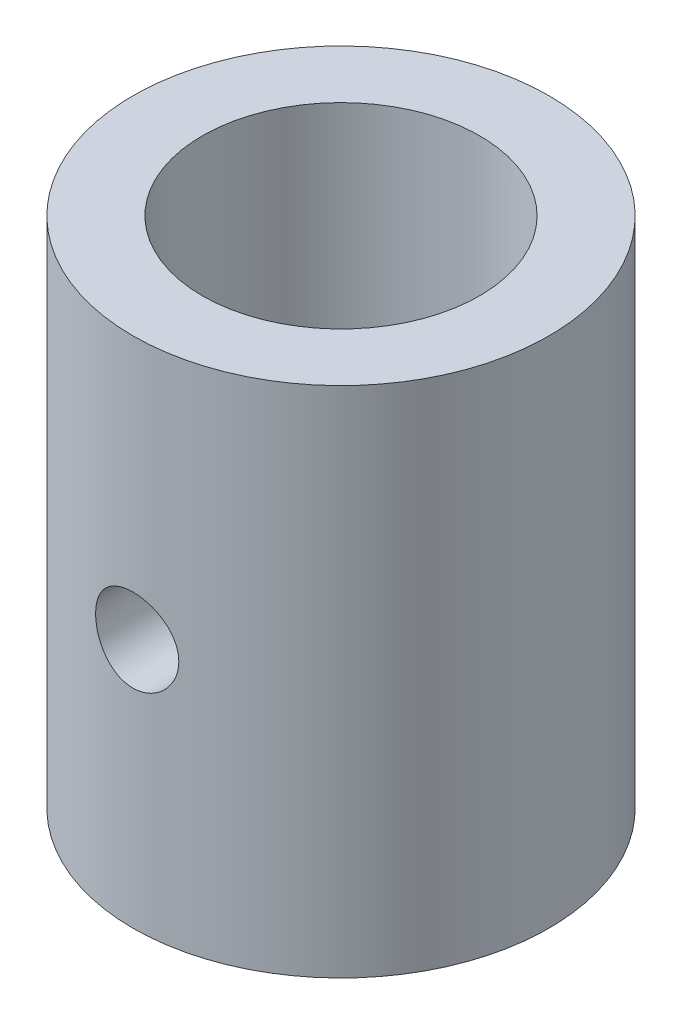
ISO-10303-21;
HEADER;
FILE_DESCRIPTION(('STEP AP214'),'2;1');
FILE_NAME('part.step','',(''),(''),'','','');
FILE_SCHEMA(('AUTOMOTIVE_DESIGN { 1 0 10303 214 1 1 1 1 }'));
ENDSEC;
DATA;
#1=APPLICATION_CONTEXT('core data for automotive mechanical design processes');
#2=APPLICATION_PROTOCOL_DEFINITION('international standard','automotive_design',2000,#1);
#3=PRODUCT_CONTEXT('',#1,'mechanical');
#4=PRODUCT('Part','Part','',(#3));
#5=PRODUCT_RELATED_PRODUCT_CATEGORY('part','',(#4));
#6=PRODUCT_DEFINITION_FORMATION('','',#4);
#7=PRODUCT_DEFINITION_CONTEXT('part definition',#1,'design');
#8=PRODUCT_DEFINITION('design','',#6,#7);
#9=PRODUCT_DEFINITION_SHAPE('','',#8);
#10=(LENGTH_UNIT() NAMED_UNIT(*) SI_UNIT(.MILLI.,.METRE.));
#11=(NAMED_UNIT(*) PLANE_ANGLE_UNIT() SI_UNIT($,.RADIAN.));
#12=(NAMED_UNIT(*) SI_UNIT($,.STERADIAN.) SOLID_ANGLE_UNIT());
#13=UNCERTAINTY_MEASURE_WITH_UNIT(LENGTH_MEASURE(1.E-05),#10,'distance_accuracy_value','');
#14=(GEOMETRIC_REPRESENTATION_CONTEXT(3) GLOBAL_UNCERTAINTY_ASSIGNED_CONTEXT((#13)) GLOBAL_UNIT_ASSIGNED_CONTEXT((#10,
#11,#12)) REPRESENTATION_CONTEXT('',''));
#15=CARTESIAN_POINT('',(0.,0.,0.));
#16=DIRECTION('',(0.,0.,1.));
#17=DIRECTION('',(1.,0.,0.));
#18=AXIS2_PLACEMENT_3D('',#15,#16,#17);
#19=CARTESIAN_POINT('',(0.,18.5,0.));
#20=DIRECTION('',(0.,1.,0.));
#21=DIRECTION('',(0.,0.,1.));
#22=AXIS2_PLACEMENT_3D('',#19,#20,#21);
#23=PLANE('',#22);
#24=CARTESIAN_POINT('',(0.,18.5,0.));
#25=DIRECTION('',(0.,1.,0.));
#26=DIRECTION('',(0.,0.,1.));
#27=AXIS2_PLACEMENT_3D('',#24,#25,#26);
#28=CIRCLE('',#27,15.);
#29=CARTESIAN_POINT('',(0.,18.5,15.));
#30=VERTEX_POINT('',#29);
#31=EDGE_CURVE('E10',#30,#30,#28,.T.);
#32=ORIENTED_EDGE('',*,*,#31,.T.);
#33=EDGE_LOOP('',(#32));
#34=FACE_BOUND('',#33,.T.);
#35=CARTESIAN_POINT('',(0.,18.5,0.));
#36=DIRECTION('',(0.,1.,0.));
#37=DIRECTION('',(0.,0.,1.));
#38=AXIS2_PLACEMENT_3D('',#35,#36,#37);
#39=CIRCLE('',#38,10.);
#40=CARTESIAN_POINT('',(0.,18.5,10.));
#41=VERTEX_POINT('',#40);
#42=EDGE_CURVE('E57',#41,#41,#39,.T.);
#43=ORIENTED_EDGE('',*,*,#42,.F.);
#44=EDGE_LOOP('',(#43));
#45=FACE_BOUND('',#44,.T.);
#46=ADVANCED_FACE('F40',(#34,#45),#23,.T.);
#47=CARTESIAN_POINT('',(0.,-18.5,0.));
#48=DIRECTION('',(0.,1.,0.));
#49=DIRECTION('',(0.,0.,1.));
#50=AXIS2_PLACEMENT_3D('',#47,#48,#49);
#51=PLANE('',#50);
#52=CARTESIAN_POINT('',(0.,-18.5,0.));
#53=DIRECTION('',(0.,1.,0.));
#54=DIRECTION('',(0.,0.,1.));
#55=AXIS2_PLACEMENT_3D('',#52,#53,#54);
#56=CIRCLE('',#55,15.);
#57=CARTESIAN_POINT('',(0.,-18.5,15.));
#58=VERTEX_POINT('',#57);
#59=EDGE_CURVE('E51',#58,#58,#56,.T.);
#60=ORIENTED_EDGE('',*,*,#59,.F.);
#61=EDGE_LOOP('',(#60));
#62=FACE_BOUND('',#61,.T.);
#63=CARTESIAN_POINT('',(0.,-18.5,0.));
#64=DIRECTION('',(0.,1.,0.));
#65=DIRECTION('',(0.,0.,1.));
#66=AXIS2_PLACEMENT_3D('',#63,#64,#65);
#67=CIRCLE('',#66,10.);
#68=CARTESIAN_POINT('',(0.,-18.5,10.));
#69=VERTEX_POINT('',#68);
#70=EDGE_CURVE('E56',#69,#69,#67,.T.);
#71=ORIENTED_EDGE('',*,*,#70,.T.);
#72=EDGE_LOOP('',(#71));
#73=FACE_BOUND('',#72,.T.);
#74=ADVANCED_FACE('F92',(#62,#73),#51,.F.);
#75=CARTESIAN_POINT('',(0.,18.5,0.));
#76=DIRECTION('',(0.,-1.,0.));
#77=DIRECTION('',(0.,0.,-1.));
#78=AXIS2_PLACEMENT_3D('',#75,#76,#77);
#79=CYLINDRICAL_SURFACE('',#78,15.);
#80=CARTESIAN_POINT('',(0.,2.5,-15.));
#81=CARTESIAN_POINT('',(-0.1667307203779,2.49999386650496,-14.9999969274261));
#82=CARTESIAN_POINT('',(-0.333538980604567,2.48605347109706,-14.9971915553469));
#83=CARTESIAN_POINT('',(-0.662440523067058,2.43070449965426,-14.9862709686969));
#84=CARTESIAN_POINT('',(-0.824529952624068,2.38927410159547,-14.9781515358056));
#85=CARTESIAN_POINT('',(-1.13919091578994,2.28027617913763,-14.9575094783486));
#86=CARTESIAN_POINT('',(-1.2917714037994,2.21273368946594,-14.9449910723015));
#87=CARTESIAN_POINT('',(-1.58342396659268,2.05350325746612,-14.9169119410594));
#88=CARTESIAN_POINT('',(-1.72249684522744,1.96181675317838,-14.9013513970712));
#89=CARTESIAN_POINT('',(-1.9850804319446,1.7555845171257,-14.8686649598991));
#90=CARTESIAN_POINT('',(-2.10838185347557,1.64077493382639,-14.8515223651304));
#91=CARTESIAN_POINT('',(-2.33411026982409,1.39212275082489,-14.8177254135776));
#92=CARTESIAN_POINT('',(-2.43653563431127,1.25827866599464,-14.8010710950127));
#93=CARTESIAN_POINT('',(-2.61849526004286,0.973851420964374,-14.7699732543785));
#94=CARTESIAN_POINT('',(-2.6978128165976,0.823127068610921,-14.7555512209484));
#95=CARTESIAN_POINT('',(-2.82991699974092,0.510154542987761,-14.7307880417525));
#96=CARTESIAN_POINT('',(-2.88270624731171,0.347907509960964,-14.7204464928588));
#97=CARTESIAN_POINT('',(-2.95957589965448,0.0187469082762474,-14.7051841575661));
#98=CARTESIAN_POINT('',(-2.98402349387633,-0.148077632426679,-14.7001941032156));
#99=CARTESIAN_POINT('',(-3.00465638317836,-0.483529464093028,-14.6959912518188));
#100=CARTESIAN_POINT('',(-3.0008445681405,-0.652156568960437,-14.6967778640352));
#101=CARTESIAN_POINT('',(-2.96536371930546,-0.98374036406301,-14.7039765344455));
#102=CARTESIAN_POINT('',(-2.93411562073172,-1.14674421688194,-14.7103035857629));
#103=CARTESIAN_POINT('',(-2.84531365386915,-1.46514822998901,-14.7277363848));
#104=CARTESIAN_POINT('',(-2.78775852930204,-1.62054802675702,-14.7388423607334));
#105=CARTESIAN_POINT('',(-2.64757435102416,-1.9205457851108,-14.7646685550122));
#106=CARTESIAN_POINT('',(-2.56477845369634,-2.06506363870752,-14.7794126944111));
#107=CARTESIAN_POINT('',(-2.37658072371804,-2.33831254991844,-14.8108385631919));
#108=CARTESIAN_POINT('',(-2.27117629307049,-2.46704179055347,-14.827520515151));
#109=CARTESIAN_POINT('',(-2.03849980368175,-2.70748820737081,-14.8613106372439));
#110=CARTESIAN_POINT('',(-1.91086848363733,-2.81885770357739,-14.8784210763271));
#111=CARTESIAN_POINT('',(-1.63855507218603,-3.01866153890367,-14.9108654614323));
#112=CARTESIAN_POINT('',(-1.49387276213817,-3.10709558388074,-14.9261993846692));
#113=CARTESIAN_POINT('',(-1.19117816063676,-3.25858252767793,-14.9534007048266));
#114=CARTESIAN_POINT('',(-1.0331454587559,-3.32159568093361,-14.9652626654482));
#115=CARTESIAN_POINT('',(-0.708446929345995,-3.4200814221157,-14.9841422696357));
#116=CARTESIAN_POINT('',(-0.541782150217349,-3.45555734622088,-14.9911605000159));
#117=CARTESIAN_POINT('',(-0.207538216881451,-3.49746936138283,-14.999480156006));
#118=CARTESIAN_POINT('',(-0.0400209849767287,-3.50438125862081,-15.0008752395741));
#119=CARTESIAN_POINT('',(0.293774802578142,-3.49025042317346,-14.9980515579031));
#120=CARTESIAN_POINT('',(0.46005342733138,-3.46920926194221,-14.9938331082434));
#121=CARTESIAN_POINT('',(0.785116979839623,-3.40016487936813,-14.9803149602405));
#122=CARTESIAN_POINT('',(0.94395584501971,-3.35240579450629,-14.9710612921262));
#123=CARTESIAN_POINT('',(1.251370882499,-3.23154805203257,-14.948506561831));
#124=CARTESIAN_POINT('',(1.39994628491262,-3.15844749596951,-14.9352051964268));
#125=CARTESIAN_POINT('',(1.68462352105865,-2.98795252804606,-14.9057973459988));
#126=CARTESIAN_POINT('',(1.82055038025656,-2.89027165688316,-14.8896585131116));
#127=CARTESIAN_POINT('',(2.07425405735762,-2.67377242637816,-14.8564420448965));
#128=CARTESIAN_POINT('',(2.19202892679229,-2.5549518008004,-14.8393643090516));
#129=CARTESIAN_POINT('',(2.40792177232253,-2.29737994432663,-14.8058791067089));
#130=CARTESIAN_POINT('',(2.50571310734597,-2.15835276733599,-14.7894858069991));
#131=CARTESIAN_POINT('',(2.67655626015362,-1.86556591592996,-14.7595257538858));
#132=CARTESIAN_POINT('',(2.74960906776871,-1.71180683127934,-14.7459588874003));
#133=CARTESIAN_POINT('',(2.86845552474588,-1.39469526155135,-14.7233022175315));
#134=CARTESIAN_POINT('',(2.91439049937315,-1.23139747636904,-14.7141892461656));
#135=CARTESIAN_POINT('',(2.97812595488159,-0.899199639527285,-14.7014231037608));
#136=CARTESIAN_POINT('',(2.99593010467534,-0.730300321371958,-14.6977692207333));
#137=CARTESIAN_POINT('',(3.00276273260241,-0.394973406367044,-14.6963744889414));
#138=CARTESIAN_POINT('',(2.99230736421269,-0.228556553218971,-14.698527575679));
#139=CARTESIAN_POINT('',(2.94405691230018,0.10009494971508,-14.7082672045384));
#140=CARTESIAN_POINT('',(2.90626204838789,0.262329633084415,-14.7158537030151));
#141=CARTESIAN_POINT('',(2.80463570549686,0.577683133721635,-14.7355579265748));
#142=CARTESIAN_POINT('',(2.74086752015203,0.730823081507248,-14.7476646305649));
#143=CARTESIAN_POINT('',(2.58916393380481,1.02431116220332,-14.7750514492251));
#144=CARTESIAN_POINT('',(2.50122650632465,1.16465822117541,-14.7903318299668));
#145=CARTESIAN_POINT('',(2.30191774435924,1.43114671645094,-14.8226688156968));
#146=CARTESIAN_POINT('',(2.19017366170554,1.55700629580279,-14.839751187291));
#147=CARTESIAN_POINT('',(1.94719310703942,1.78835861658751,-14.8735824561586));
#148=CARTESIAN_POINT('',(1.81595216146,1.89384667095182,-14.8903312758955));
#149=CARTESIAN_POINT('',(1.53605288726474,2.08250393183934,-14.9218149716391));
#150=CARTESIAN_POINT('',(1.3872266532895,2.16542800984008,-14.9365269365774));
#151=CARTESIAN_POINT('',(1.0774990828222,2.30495836778978,-14.96205375255));
#152=CARTESIAN_POINT('',(0.916608782589378,2.36158836859748,-14.9728721141585));
#153=CARTESIAN_POINT('',(0.629464466771338,2.43595584413415,-14.9872911778611));
#154=CARTESIAN_POINT('',(0.504844992041353,2.45992958112327,-14.9920290947535));
#155=CARTESIAN_POINT('',(0.253498575630201,2.49195373707509,-14.9983846241968));
#156=CARTESIAN_POINT('',(0.126771701245857,2.5000046635293,-15.0000023361946));
#157=CARTESIAN_POINT('',(0.,2.5,-15.));
#158=B_SPLINE_CURVE_WITH_KNOTS('',3,(#80,#81,#82,#83,#84,#85,#86,#87,#88,#89,#90,#91,#92,#93,
#94,#95,#96,#97,#98,#99,#100,#101,#102,#103,#104,#105,#106,#107,#108,#109,#110,#111,#112,#113,
#114,#115,#116,#117,#118,#119,#120,#121,#122,#123,#124,#125,#126,#127,#128,#129,#130,#131,#132,
#133,#134,#135,#136,#137,#138,#139,#140,#141,#142,#143,#144,#145,#146,#147,#148,#149,#150,#151,
#152,#153,#154,#155,#156,#157),.UNSPECIFIED.,.T.,.F.,(4,2,2,2,2,2,2,2,2,2,2,2,2,2,2,2,2,2,2,2,2,
2,2,2,2,2,2,2,2,2,2,2,2,2,2,2,2,2,4),(0.,0.499728391983776,0.999853952073969,1.49950120575102,
1.99911870669259,2.50479801033656,3.0105167902421,3.52083585017768,4.03110448095592,
4.53468555310762,5.03821512843675,5.53415181018835,6.03011217761189,6.52942470610778,
7.02879464249011,7.53714757474052,8.04550702619461,8.55465824562072,9.06374777094108,
9.56432207028796,10.064868229736,10.5609136185217,11.0569961764807,11.5591519810008,
12.0613616503779,12.5712188573768,13.081055661704,13.5882114309817,14.0953010499124,
14.593191677031,15.0910783047783,15.5877588375933,16.084481027456,16.5896422871743,
17.0949196359879,17.6054849002691,18.1155886655256,18.4955632586968,18.8755257411299),.UNSPECIFIED.);
#159=CARTESIAN_POINT('',(0.,2.5,-15.));
#160=VERTEX_POINT('',#159);
#161=EDGE_CURVE('E83',#160,#160,#158,.T.);
#162=ORIENTED_EDGE('',*,*,#161,.T.);
#163=EDGE_LOOP('',(#162));
#164=FACE_BOUND('',#163,.T.);
#165=CARTESIAN_POINT('',(3.,-0.5,14.6969384566991));
#166=CARTESIAN_POINT('',(2.99999383762581,-0.666693126473467,14.6969417707994));
#167=CARTESIAN_POINT('',(2.98605951515443,-0.833463870000021,14.6998052480611));
#168=CARTESIAN_POINT('',(2.93073685074852,-1.1622875154294,14.7109329391462));
#169=CARTESIAN_POINT('',(2.88932654121148,-1.32433653390794,14.7192014743436));
#170=CARTESIAN_POINT('',(2.78038734785924,-1.63891191006263,14.7401662116556));
#171=CARTESIAN_POINT('',(2.71288444245786,-1.79144756459777,14.7528580086323));
#172=CARTESIAN_POINT('',(2.55374732301152,-2.08302453409087,14.7812339844198));
#173=CARTESIAN_POINT('',(2.46211445580345,-2.22206660161371,14.7969179962038));
#174=CARTESIAN_POINT('',(2.25593722696031,-2.48468301156158,14.8297589908276));
#175=CARTESIAN_POINT('',(2.14111696773996,-2.60803876365192,14.8469321351174));
#176=CARTESIAN_POINT('',(1.89242036706393,-2.83387260073694,14.880674169078));
#177=CARTESIAN_POINT('',(1.75854269093395,-2.93634922225158,14.8972430163249));
#178=CARTESIAN_POINT('',(1.47408406777277,-3.11836405288538,14.9280838925269));
#179=CARTESIAN_POINT('',(1.32336770301663,-3.19769454144992,14.9423346432465));
#180=CARTESIAN_POINT('',(1.01041245116182,-3.32982481114441,14.9667521065089));
#181=CARTESIAN_POINT('',(0.84817464426166,-3.38262707570297,14.9769192013236));
#182=CARTESIAN_POINT('',(0.519050319835483,-3.45952158085887,14.9919096206526));
#183=CARTESIAN_POINT('',(0.352253217644443,-3.48398293271302,14.9968015886438));
#184=CARTESIAN_POINT('',(0.0168557053126099,-3.50465285551495,15.0009276355081));
#185=CARTESIAN_POINT('',(-0.151744529495528,-3.50086414893747,15.0001622595828));
#186=CARTESIAN_POINT('',(-0.483426002230765,-3.46542145935334,14.9931130460555));
#187=CARTESIAN_POINT('',(-0.646551642895409,-3.43416506849646,14.9869079509751));
#188=CARTESIAN_POINT('',(-0.965194879740902,-3.34530490262332,14.9697653147823));
#189=CARTESIAN_POINT('',(-1.12071217124139,-3.28770007342438,14.9588275843212));
#190=CARTESIAN_POINT('',(-1.42085838960266,-3.1474098795582,14.9333188805988));
#191=CARTESIAN_POINT('',(-1.5654125224017,-3.06456874668534,14.9187254452567));
#192=CARTESIAN_POINT('',(-1.83871513757927,-2.8762727682902,14.8875140842136));
#193=CARTESIAN_POINT('',(-1.967461798575,-2.77081532068845,14.8708959256567));
#194=CARTESIAN_POINT('',(-2.20785429316037,-2.53809913367458,14.8371289309338));
#195=CARTESIAN_POINT('',(-2.31916294972089,-2.41049243981123,14.8199758937255));
#196=CARTESIAN_POINT('',(-2.51885547953042,-2.13825067264774,14.7873471479628));
#197=CARTESIAN_POINT('',(-2.60723891918325,-1.99361527735041,14.7718714711364));
#198=CARTESIAN_POINT('',(-2.75868844440564,-1.69093750453459,14.7443414241877));
#199=CARTESIAN_POINT('',(-2.82169994333313,-1.53286709708102,14.7322944469065));
#200=CARTESIAN_POINT('',(-2.92017102488275,-1.20808602882803,14.7130942896382));
#201=CARTESIAN_POINT('',(-2.95563419836993,-1.04137649714275,14.7059404718528));
#202=CARTESIAN_POINT('',(-2.99749801810815,-0.707105426002867,14.6974643780348));
#203=CARTESIAN_POINT('',(-3.00438557669374,-0.539607277068979,14.6960444117146));
#204=CARTESIAN_POINT('',(-2.99021288493222,-0.20585533040095,14.6989345706656));
#205=CARTESIAN_POINT('',(-2.96915421936733,-0.0396014626434112,14.7032443710116));
#206=CARTESIAN_POINT('',(-2.90010662422247,0.285305920876705,14.7170169748474));
#207=CARTESIAN_POINT('',(-2.8523778625179,0.444017029107287,14.7264299704349));
#208=CARTESIAN_POINT('',(-2.73162310592555,0.751189837086223,14.7493046805499));
#209=CARTESIAN_POINT('',(-2.65859502711953,0.89965069130716,14.7627667285881));
#210=CARTESIAN_POINT('',(-2.48821242664679,1.18423932985048,14.7924421788612));
#211=CARTESIAN_POINT('',(-2.39055323394826,1.32018113890248,14.8086891559471));
#212=CARTESIAN_POINT('',(-2.17408671663814,1.57392493600274,14.8420117147991));
#213=CARTESIAN_POINT('',(-2.05527721543361,1.69172505474776,14.8590873817145));
#214=CARTESIAN_POINT('',(-1.79769682049367,1.90768767755673,14.8924603760765));
#215=CARTESIAN_POINT('',(-1.65864749678889,2.00552096394999,14.9087417312605));
#216=CARTESIAN_POINT('',(-1.36580368990427,2.17643764449875,14.9384138288586));
#217=CARTESIAN_POINT('',(-1.21200982630052,2.24952207803435,14.9518046926563));
#218=CARTESIAN_POINT('',(-0.894908042472039,2.3683866152399,14.974118821832));
#219=CARTESIAN_POINT('',(-0.731660020434235,2.41432155467876,14.9830673742781));
#220=CARTESIAN_POINT('',(-0.399568364039735,2.47807374299153,14.9955970781298));
#221=CARTESIAN_POINT('',(-0.230725406133636,2.49589437842704,14.9991788759955));
#222=CARTESIAN_POINT('',(0.104618681710863,2.50278094288867,15.0005562136234));
#223=CARTESIAN_POINT('',(0.271109436424482,2.49234184136868,14.9984513564799));
#224=CARTESIAN_POINT('',(0.599913093946949,2.44409814835652,14.9889013068102));
#225=CARTESIAN_POINT('',(0.762226049261167,2.40629390095561,14.9814561814329));
#226=CARTESIAN_POINT('',(1.07775824923519,2.30461302372524,14.9620649509476));
#227=CARTESIAN_POINT('',(1.23099732972049,2.24079586560708,14.9501291174284));
#228=CARTESIAN_POINT('',(1.52466366055821,2.08896327600667,14.9230416637104));
#229=CARTESIAN_POINT('',(1.66508989730354,2.0009459322865,14.9078897894096));
#230=CARTESIAN_POINT('',(1.93159167031775,1.80154183881615,14.8757279747022));
#231=CARTESIAN_POINT('',(2.05739914834453,1.68980099084868,14.858692002537));
#232=CARTESIAN_POINT('',(2.28864785327552,1.44684927970369,14.8248366872359));
#233=CARTESIAN_POINT('',(2.39408424962674,1.31563381156023,14.8080173963616));
#234=CARTESIAN_POINT('',(2.58267665834994,1.03576204992871,14.7763002820179));
#235=CARTESIAN_POINT('',(2.66558044385427,0.886933116636243,14.7614251071368));
#236=CARTESIAN_POINT('',(2.80507214779868,0.577201680219698,14.7355571137924));
#237=CARTESIAN_POINT('',(2.86168393792249,0.416310283938431,14.7245607757495));
#238=CARTESIAN_POINT('',(2.93600741957297,0.129212633671379,14.7098904341354));
#239=CARTESIAN_POINT('',(2.95996169557105,0.00464374145812644,14.7050635474382));
#240=CARTESIAN_POINT('',(2.99196005387913,-0.246601863653405,14.6985863537725));
#241=CARTESIAN_POINT('',(3.00000468468793,-0.373278503733406,14.6969359372925));
#242=CARTESIAN_POINT('',(3.,-0.5,14.6969384566991));
#243=B_SPLINE_CURVE_WITH_KNOTS('',3,(#165,#166,#167,#168,#169,#170,#171,#172,#173,#174,#175,
#176,#177,#178,#179,#180,#181,#182,#183,#184,#185,#186,#187,#188,#189,#190,#191,#192,#193,#194,
#195,#196,#197,#198,#199,#200,#201,#202,#203,#204,#205,#206,#207,#208,#209,#210,#211,#212,#213,
#214,#215,#216,#217,#218,#219,#220,#221,#222,#223,#224,#225,#226,#227,#228,#229,#230,#231,#232,
#233,#234,#235,#236,#237,#238,#239,#240,#241,#242),.UNSPECIFIED.,.T.,.F.,(4,2,2,2,2,2,2,2,2,2,2,
2,2,2,2,2,2,2,2,2,2,2,2,2,2,2,2,2,2,2,2,2,2,2,2,2,2,2,4),(0.,0.499615391608283,0.99963071785289,
1.49914949382176,1.99864039457959,2.5044675764531,3.01033020106266,3.52060201312351,
4.03082604739679,4.53432746649241,5.03778036348745,5.53406368900612,6.03036687221251,
6.5297977266691,7.02928607310198,7.5374804028745,8.04568434368161,8.5549758951833,
9.06420105048074,9.56471273413781,10.0651960358526,10.5608802534996,11.056605310632,
11.5587917932356,12.0610299861063,12.5709780520035,13.0809046989031,13.5878944073595,
14.0948230407488,14.5929305224406,15.0910317410027,15.5880005122636,16.0850085640405,
16.5900345607679,17.0951801666934,17.6057669573882,18.1158892527059,18.4957141091448,
18.8755258705644),.UNSPECIFIED.);
#244=CARTESIAN_POINT('',(3.,-0.5,14.6969384566991));
#245=VERTEX_POINT('',#244);
#246=EDGE_CURVE('E78',#245,#245,#243,.T.);
#247=ORIENTED_EDGE('',*,*,#246,.T.);
#248=EDGE_LOOP('',(#247));
#249=FACE_BOUND('',#248,.T.);
#250=ORIENTED_EDGE('',*,*,#31,.F.);
#251=EDGE_LOOP('',(#250));
#252=FACE_BOUND('',#251,.T.);
#253=ORIENTED_EDGE('',*,*,#59,.T.);
#254=EDGE_LOOP('',(#253));
#255=FACE_BOUND('',#254,.T.);
#256=ADVANCED_FACE('F39',(#164,#249,#252,#255),#79,.T.);
#257=CARTESIAN_POINT('',(0.,18.5,0.));
#258=DIRECTION('',(0.,-1.,0.));
#259=DIRECTION('',(0.,0.,-1.));
#260=AXIS2_PLACEMENT_3D('',#257,#258,#259);
#261=CYLINDRICAL_SURFACE('',#260,10.);
#262=CARTESIAN_POINT('',(0.,2.5,-10.));
#263=CARTESIAN_POINT('',(-0.1645772255066,2.49999800503023,-9.99999858501101));
#264=CARTESIAN_POINT('',(-0.329174636703059,2.48641227275207,-9.99589831387907));
#265=CARTESIAN_POINT('',(-0.653576250609762,2.4325572915558,-9.97994211187382));
#266=CARTESIAN_POINT('',(-0.81337900882284,2.39228008395331,-9.96808386779384));
#267=CARTESIAN_POINT('',(-1.12346541550905,2.28650796617947,-9.93791105003673));
#268=CARTESIAN_POINT('',(-1.27376272879075,2.22105026076213,-9.91960600500851));
#269=CARTESIAN_POINT('',(-1.56124836210626,2.06692781388833,-9.87844218475291));
#270=CARTESIAN_POINT('',(-1.69843493493934,1.97825998520917,-9.85558280384133));
#271=CARTESIAN_POINT('',(-1.95974359436749,1.77755198505466,-9.80701474385548));
#272=CARTESIAN_POINT('',(-2.08343614248868,1.66496674822817,-9.78124767314073));
#273=CARTESIAN_POINT('',(-2.31049841846647,1.42078154017963,-9.73011668420884));
#274=CARTESIAN_POINT('',(-2.41386472654882,1.28917837575008,-9.70475283449003));
#275=CARTESIAN_POINT('',(-2.59960075447415,1.00705849392478,-9.65668227987544));
#276=CARTESIAN_POINT('',(-2.68144618044427,0.856183078018524,-9.63404813327749));
#277=CARTESIAN_POINT('',(-2.81842789549521,0.542021491539414,-9.59487240788062));
#278=CARTESIAN_POINT('',(-2.87357059839947,0.378738312144048,-9.57832936626621));
#279=CARTESIAN_POINT('',(-2.95403267365303,0.0492194677390801,-9.55381741676868));
#280=CARTESIAN_POINT('',(-2.98014392469355,-0.116805487727887,-9.54562138649067));
#281=CARTESIAN_POINT('',(-3.00427461229344,-0.451066312433532,-9.53805579499534));
#282=CARTESIAN_POINT('',(-3.00230085522157,-0.619301636118176,-9.53868409521142));
#283=CARTESIAN_POINT('',(-2.97093954399623,-0.946767817216969,-9.54849488135555));
#284=CARTESIAN_POINT('',(-2.9425441052537,-1.10610450072448,-9.55736777198281));
#285=CARTESIAN_POINT('',(-2.86074840854112,-1.41763957254692,-9.58216712457248));
#286=CARTESIAN_POINT('',(-2.80734568283282,-1.56983725474867,-9.59809428264701));
#287=CARTESIAN_POINT('',(-2.67632053307363,-1.86520069932148,-9.63545466149946));
#288=CARTESIAN_POINT('',(-2.59837633869285,-2.00821416791053,-9.65696032231904));
#289=CARTESIAN_POINT('',(-2.42070445177367,-2.27946404402039,-9.70301974000129));
#290=CARTESIAN_POINT('',(-2.32097148005177,-2.40769685882756,-9.72757423493982));
#291=CARTESIAN_POINT('',(-2.09762581531093,-2.65137238152404,-9.77822022595875));
#292=CARTESIAN_POINT('',(-1.97318981493394,-2.76605732805934,-9.80433308620996));
#293=CARTESIAN_POINT('',(-1.70652651862793,-2.9731079681285,-9.85424488126517));
#294=CARTESIAN_POINT('',(-1.56429810372178,-3.06547225682885,-9.8780436703682));
#295=CARTESIAN_POINT('',(-1.26471007668561,-3.22571984492946,-9.92086320138941));
#296=CARTESIAN_POINT('',(-1.1072554994959,-3.29343503249972,-9.93985087336628));
#297=CARTESIAN_POINT('',(-0.782490831207038,-3.40119918019926,-9.97067043664444));
#298=CARTESIAN_POINT('',(-0.615183503179163,-3.44125585706498,-9.98250432373999));
#299=CARTESIAN_POINT('',(-0.281904485336663,-3.49130435579879,-9.99736729287077));
#300=CARTESIAN_POINT('',(-0.116100195202374,-3.50232317160322,-10.0006970083558));
#301=CARTESIAN_POINT('',(0.214999211646766,-3.49686168857584,-9.99905846483519));
#302=CARTESIAN_POINT('',(0.380294393381561,-3.48038506069712,-9.99409131355514));
#303=CARTESIAN_POINT('',(0.701807210619393,-3.42123077777701,-9.97661393974325));
#304=CARTESIAN_POINT('',(0.858145545228338,-3.37915322483826,-9.96427659598829));
#305=CARTESIAN_POINT('',(1.16150927790904,-3.2707135344436,-9.9334869568307));
#306=CARTESIAN_POINT('',(1.30853355405117,-3.20434847792428,-9.91503392642188));
#307=CARTESIAN_POINT('',(1.5928743789221,-3.04749366903774,-9.87339308702631));
#308=CARTESIAN_POINT('',(1.72988765239933,-2.95648131810404,-9.8501056165928));
#309=CARTESIAN_POINT('',(1.9870466159603,-2.75355049189439,-9.80146937528705));
#310=CARTESIAN_POINT('',(2.10718806471188,-2.6416267762247,-9.7761200886242));
#311=CARTESIAN_POINT('',(2.33171489102052,-2.39522538326126,-9.72506343738007));
#312=CARTESIAN_POINT('',(2.43536962463001,-2.26007624845635,-9.69937650065513));
#313=CARTESIAN_POINT('',(2.61857990144313,-1.97374412197312,-9.65153030477949));
#314=CARTESIAN_POINT('',(2.69813607658965,-1.82256155088424,-9.62937095313121));
#315=CARTESIAN_POINT('',(2.83034694254316,-1.50893501748996,-9.5913437922631));
#316=CARTESIAN_POINT('',(2.88312693874022,-1.34654762692434,-9.575446756735));
#317=CARTESIAN_POINT('',(2.96043461630306,-1.01462406213953,-9.55183188739737));
#318=CARTESIAN_POINT('',(2.98497197957849,-0.845090358433927,-9.54411125069387));
#319=CARTESIAN_POINT('',(3.0044396896993,-0.511276963223158,-9.53799944941558));
#320=CARTESIAN_POINT('',(3.00056110615887,-0.347072697901157,-9.53923294700394));
#321=CARTESIAN_POINT('',(2.9661501088861,-0.0217717931987715,-9.54998802392188));
#322=CARTESIAN_POINT('',(2.93561876249408,0.139324970361023,-9.55950927135902));
#323=CARTESIAN_POINT('',(2.84953777608686,0.451890798263347,-9.58551527389243));
#324=CARTESIAN_POINT('',(2.79430351014248,0.603454574717388,-9.60191209104934));
#325=CARTESIAN_POINT('',(2.66063014242147,0.895284877641445,-9.63980557805265));
#326=CARTESIAN_POINT('',(2.58218659925722,1.03554923528315,-9.6613032238508));
#327=CARTESIAN_POINT('',(2.40097527610175,1.30632623305253,-9.70795352855338));
#328=CARTESIAN_POINT('',(2.29742552185996,1.43629752252037,-9.7332108032858));
#329=CARTESIAN_POINT('',(2.07034869259555,1.67740499661618,-9.78402640899066));
#330=CARTESIAN_POINT('',(1.94681643426898,1.78853627893564,-9.80958481647543));
#331=CARTESIAN_POINT('',(1.67893152436652,1.99204682458993,-9.85901873141573));
#332=CARTESIAN_POINT('',(1.53407577158122,2.08378289371094,-9.88282319531421));
#333=CARTESIAN_POINT('',(1.23028274796705,2.24147033980808,-9.92521360911553));
#334=CARTESIAN_POINT('',(1.07135210599791,2.30743377654903,-9.94380199862114));
#335=CARTESIAN_POINT('',(0.761515425310564,2.40579055130549,-9.97204349938619));
#336=CARTESIAN_POINT('',(0.611573923908469,2.44102334576649,-9.9824405476214));
#337=CARTESIAN_POINT('',(0.307760390461558,2.48812705048316,-9.9964188898898));
#338=CARTESIAN_POINT('',(0.153889019716279,2.50000186540964,-10.0000013230948));
#339=CARTESIAN_POINT('',(0.,2.5,-10.));
#340=B_SPLINE_CURVE_WITH_KNOTS('',3,(#262,#263,#264,#265,#266,#267,#268,#269,#270,#271,#272,
#273,#274,#275,#276,#277,#278,#279,#280,#281,#282,#283,#284,#285,#286,#287,#288,#289,#290,#291,
#292,#293,#294,#295,#296,#297,#298,#299,#300,#301,#302,#303,#304,#305,#306,#307,#308,#309,#310,
#311,#312,#313,#314,#315,#316,#317,#318,#319,#320,#321,#322,#323,#324,#325,#326,#327,#328,#329,
#330,#331,#332,#333,#334,#335,#336,#337,#338,#339),.UNSPECIFIED.,.T.,.F.,(4,2,2,2,2,2,2,2,2,2,2,
2,2,2,2,2,2,2,2,2,2,2,2,2,2,2,2,2,2,2,2,2,2,2,2,2,2,2,4),(0.,0.493166407225221,
0.986479929691999,1.47906735260175,1.9717203288254,2.47711205896383,2.98258874577266,
3.49942962008218,4.01614629086447,4.51839378713198,5.02051956638179,5.50452033395352,
5.98856887316002,6.47924852894239,6.97004720317111,7.48134208096333,7.99266913062143,
8.50742093763377,9.02202907057615,9.5181761887709,10.0142570710065,10.4991349336465,
10.9840710918746,11.4802261140582,11.9765056400038,12.4908080064564,13.0050968850536,
13.516956299025,14.0286401892057,14.5190031093854,15.0093463933232,15.4936008081456,
15.9779479511533,16.4799385136898,16.9820594980412,17.4988599232246,18.0154182319959,
18.4766338387004,18.9377723390687),.UNSPECIFIED.);
#341=CARTESIAN_POINT('',(0.,2.5,-10.));
#342=VERTEX_POINT('',#341);
#343=EDGE_CURVE('E45',#342,#342,#340,.T.);
#344=ORIENTED_EDGE('',*,*,#343,.F.);
#345=EDGE_LOOP('',(#344));
#346=FACE_BOUND('',#345,.T.);
#347=CARTESIAN_POINT('',(3.,-0.5,9.53939201416946));
#348=CARTESIAN_POINT('',(2.99999795267528,-0.664389095884808,9.5393937145396));
#349=CARTESIAN_POINT('',(2.98644216334284,-0.82879844828805,9.54368780418137));
#350=CARTESIAN_POINT('',(2.93271688893498,-1.15281049918389,9.56033156605799));
#351=CARTESIAN_POINT('',(2.89253851147156,-1.31241157300293,9.57268392986936));
#352=CARTESIAN_POINT('',(2.78705506539911,-1.62206945654346,9.60392204971265));
#353=CARTESIAN_POINT('',(2.72179178788487,-1.77214165926617,9.62279693406464));
#354=CARTESIAN_POINT('',(2.56812843835858,-2.0592438679906,9.66493865095134));
#355=CARTESIAN_POINT('',(2.47972490274105,-2.19627191736888,9.68820614082039));
#356=CARTESIAN_POINT('',(2.27929508283254,-2.45773278115475,9.73733724371531));
#357=CARTESIAN_POINT('',(2.16666414351613,-2.58169179589258,9.76325616623271));
#358=CARTESIAN_POINT('',(1.9222724751592,-2.80927590264502,9.81429723873514));
#359=CARTESIAN_POINT('',(1.79050929092222,-2.91289838089976,9.8394192859541));
#360=CARTESIAN_POINT('',(1.50822287558738,-3.09892539966661,9.88666429158777));
#361=CARTESIAN_POINT('',(1.35736804267163,-3.18084684888562,9.90871448684808));
#362=CARTESIAN_POINT('',(1.04324929073871,-3.31797451808551,9.94668871841369));
#363=CARTESIAN_POINT('',(0.879988056775823,-3.3731864997149,9.96261407578992));
#364=CARTESIAN_POINT('',(0.55064770526166,-3.45376000218102,9.98615292007178));
#365=CARTESIAN_POINT('',(0.384782797907603,-3.47993025530541,9.99399114738673));
#366=CARTESIAN_POINT('',(0.0508436474986283,-3.50423464929288,10.001264030027));
#367=CARTESIAN_POINT('',(-0.117230124100743,-3.50237467880391,10.0007004504217));
#368=CARTESIAN_POINT('',(-0.445142313200314,-3.47121426291397,9.99139207635305));
#369=CARTESIAN_POINT('',(-0.60507253528266,-3.4427896123803,9.98290840410475));
#370=CARTESIAN_POINT('',(-0.917778426885076,-3.36073732801138,9.95903044225231));
#371=CARTESIAN_POINT('',(-1.07055364264578,-3.3071080981145,9.9436357150134));
#372=CARTESIAN_POINT('',(-1.36669465270248,-3.17557595316304,9.90730441973756));
#373=CARTESIAN_POINT('',(-1.50993012938864,-3.09739759438606,9.88630539352772));
#374=CARTESIAN_POINT('',(-1.78152934756663,-2.91920429514295,9.84099281296778));
#375=CARTESIAN_POINT('',(-1.90988954974545,-2.81918417407083,9.81667847277943));
#376=CARTESIAN_POINT('',(-2.15332096305837,-2.5956044984991,9.76623100973852));
#377=CARTESIAN_POINT('',(-2.26768916079755,-2.47128616194922,9.74006390633503));
#378=CARTESIAN_POINT('',(-2.47415303080115,-2.2049799642112,9.68967959784414));
#379=CARTESIAN_POINT('',(-2.56624648967452,-2.06299034918903,9.66546258669242));
#380=CARTESIAN_POINT('',(-2.72627990669511,-1.76352106152783,9.62155806359712));
#381=CARTESIAN_POINT('',(-2.79397978469378,-1.60590590838251,9.60191621258491));
#382=CARTESIAN_POINT('',(-2.90166725750739,-1.2807855832214,9.5699278496379));
#383=CARTESIAN_POINT('',(-2.94166389279494,-1.11328365696495,9.55757895796639));
#384=CARTESIAN_POINT('',(-2.99149540565762,-0.779835278497565,9.54209699116239));
#385=CARTESIAN_POINT('',(-3.00239892760807,-0.614063552205647,9.53863757349917));
#386=CARTESIAN_POINT('',(-2.99671894465741,-0.283054199986657,9.54042384874812));
#387=CARTESIAN_POINT('',(-2.98013928742559,-0.117816502539997,9.54566832310787));
#388=CARTESIAN_POINT('',(-2.92091527148479,0.202976755943388,9.56395117112153));
#389=CARTESIAN_POINT('',(-2.87895922862587,0.358672328527488,9.57678353015602));
#390=CARTESIAN_POINT('',(-2.77097155495853,0.660803381629392,9.6085828246183));
#391=CARTESIAN_POINT('',(-2.70493620685512,0.807237428281019,9.62755070717977));
#392=CARTESIAN_POINT('',(-2.54863742393008,1.09103492814438,9.67011670046268));
#393=CARTESIAN_POINT('',(-2.4577712834546,1.22804944197162,9.69382542139644));
#394=CARTESIAN_POINT('',(-2.25510603200767,1.48527621236157,9.74296411293928));
#395=CARTESIAN_POINT('',(-2.14330191069793,1.60548443522557,9.76839449459994));
#396=CARTESIAN_POINT('',(-1.8969102649872,1.83036081162948,9.81927267096329));
#397=CARTESIAN_POINT('',(-1.76162213171487,1.93427125797397,9.84468490126011));
#398=CARTESIAN_POINT('',(-1.4749235691805,2.1179334020555,9.89169703497298));
#399=CARTESIAN_POINT('',(-1.32351394108789,2.19768629956292,9.91329712769433));
#400=CARTESIAN_POINT('',(-1.00987100941044,2.33000006113659,9.95011940949915));
#401=CARTESIAN_POINT('',(-0.847729244075677,2.38276403231795,9.96538906849932));
#402=CARTESIAN_POINT('',(-0.516339933009175,2.46012183778084,9.98803959193653));
#403=CARTESIAN_POINT('',(-0.347094434709524,2.48472373189683,9.9954227134176));
#404=CARTESIAN_POINT('',(-0.0133043077654851,2.504446088109,10.001330881628));
#405=CARTESIAN_POINT('',(0.151170358172414,2.50066539081567,10.0001861022264));
#406=CARTESIAN_POINT('',(0.477038962328808,2.46635673500176,9.98994528930073));
#407=CARTESIAN_POINT('',(0.638433074693058,2.43583029303912,9.98084970660925));
#408=CARTESIAN_POINT('',(0.951871626082717,2.34957667720075,9.95582336716653));
#409=CARTESIAN_POINT('',(1.10399785470278,2.29412363870197,9.93996705801731));
#410=CARTESIAN_POINT('',(1.39686647550411,2.15983617098562,9.903058860789));
#411=CARTESIAN_POINT('',(1.53760699210116,2.08099789942762,9.88200611899892));
#412=CARTESIAN_POINT('',(1.80860378484113,1.89925308513993,9.83607931656457));
#413=CARTESIAN_POINT('',(1.93838050015354,1.79565713999847,9.81110453847119));
#414=CARTESIAN_POINT('',(2.17907514269189,1.5685792233344,9.76047074424668));
#415=CARTESIAN_POINT('',(2.28998761920387,1.4450915242037,9.73481153282158));
#416=CARTESIAN_POINT('',(2.49312538789097,1.17731844337898,9.68481361262638));
#417=CARTESIAN_POINT('',(2.58469519515913,1.03252289321912,9.66053705386971));
#418=CARTESIAN_POINT('',(2.74208627057551,0.728889651677958,9.61705095017586));
#419=CARTESIAN_POINT('',(2.80791991114577,0.570058752797607,9.59783897193911));
#420=CARTESIAN_POINT('',(2.90603885065899,0.260519136787451,9.56855633435189));
#421=CARTESIAN_POINT('',(2.94117718022463,0.110782706138014,9.5577230968104));
#422=CARTESIAN_POINT('',(2.98815637670288,-0.192630444991546,9.54314085194333));
#423=CARTESIAN_POINT('',(3.00000191412191,-0.346306369290496,9.53939042442861));
#424=CARTESIAN_POINT('',(3.,-0.5,9.53939201416946));
#425=B_SPLINE_CURVE_WITH_KNOTS('',3,(#347,#348,#349,#350,#351,#352,#353,#354,#355,#356,#357,
#358,#359,#360,#361,#362,#363,#364,#365,#366,#367,#368,#369,#370,#371,#372,#373,#374,#375,#376,
#377,#378,#379,#380,#381,#382,#383,#384,#385,#386,#387,#388,#389,#390,#391,#392,#393,#394,#395,
#396,#397,#398,#399,#400,#401,#402,#403,#404,#405,#406,#407,#408,#409,#410,#411,#412,#413,#414,
#415,#416,#417,#418,#419,#420,#421,#422,#423,#424),.UNSPECIFIED.,.T.,.F.,(4,2,2,2,2,2,2,2,2,2,2,
2,2,2,2,2,2,2,2,2,2,2,2,2,2,2,2,2,2,2,2,2,2,2,2,2,2,2,4),(0.,0.492600331831085,0.985365283378,
1.47731282893239,1.9693340507402,2.47546300015968,2.98165695742546,3.49831878547289,
4.01486911175754,4.51664280299115,5.01831108202881,5.5040025198176,5.98972471780752,
6.48110418671353,6.97260033181661,7.48304294046556,7.99353624983726,8.50892476494934,
9.02414501262032,9.52016161585828,10.0161087821998,10.4991718988284,10.9823096209678,
11.4784146362399,11.9746385186306,12.4895901220641,13.0045161465361,13.5155078363386,
14.0263532464857,14.5175260782765,15.0086710610072,15.4945419374965,15.9804926898797,
16.4819925411419,16.9836370526499,17.500232793435,18.016579879331,18.477223077201,
18.9377739007233),.UNSPECIFIED.);
#426=CARTESIAN_POINT('',(3.,-0.5,9.53939201416946));
#427=VERTEX_POINT('',#426);
#428=EDGE_CURVE('E64',#427,#427,#425,.T.);
#429=ORIENTED_EDGE('',*,*,#428,.F.);
#430=EDGE_LOOP('',(#429));
#431=FACE_BOUND('',#430,.T.);
#432=ORIENTED_EDGE('',*,*,#42,.T.);
#433=EDGE_LOOP('',(#432));
#434=FACE_BOUND('',#433,.T.);
#435=ORIENTED_EDGE('',*,*,#70,.F.);
#436=EDGE_LOOP('',(#435));
#437=FACE_BOUND('',#436,.T.);
#438=ADVANCED_FACE('F66',(#346,#431,#434,#437),#261,.F.);
#439=CARTESIAN_POINT('',(0.,-0.5,-18.5));
#440=DIRECTION('',(0.,0.,1.));
#441=DIRECTION('',(1.,0.,0.));
#442=AXIS2_PLACEMENT_3D('',#439,#440,#441);
#443=CYLINDRICAL_SURFACE('',#442,3.);
#444=ORIENTED_EDGE('',*,*,#428,.T.);
#445=EDGE_LOOP('',(#444));
#446=FACE_BOUND('',#445,.T.);
#447=ORIENTED_EDGE('',*,*,#246,.F.);
#448=EDGE_LOOP('',(#447));
#449=FACE_BOUND('',#448,.T.);
#450=ADVANCED_FACE('F75',(#446,#449),#443,.F.);
#451=ORIENTED_EDGE('',*,*,#343,.T.);
#452=EDGE_LOOP('',(#451));
#453=FACE_BOUND('',#452,.T.);
#454=ORIENTED_EDGE('',*,*,#161,.F.);
#455=EDGE_LOOP('',(#454));
#456=FACE_BOUND('',#455,.T.);
#457=ADVANCED_FACE('F68',(#453,#456),#443,.F.);
#458=CLOSED_SHELL('',(#46,#74,#256,#438,#450,#457));
#459=MANIFOLD_SOLID_BREP('B2',#458);
#460=ADVANCED_BREP_SHAPE_REPRESENTATION('',(#18,#459),#14);
#461=SHAPE_DEFINITION_REPRESENTATION(#9,#460);
ENDSEC;
END-ISO-10303-21;
